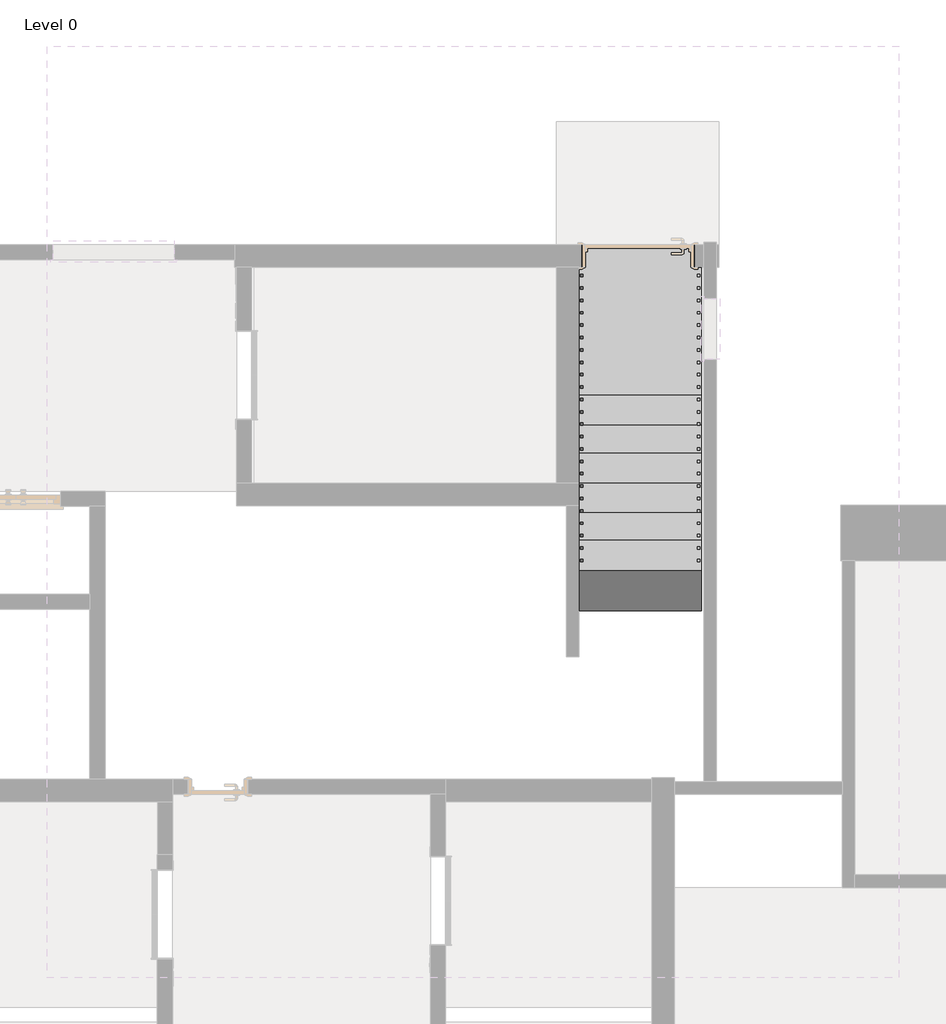
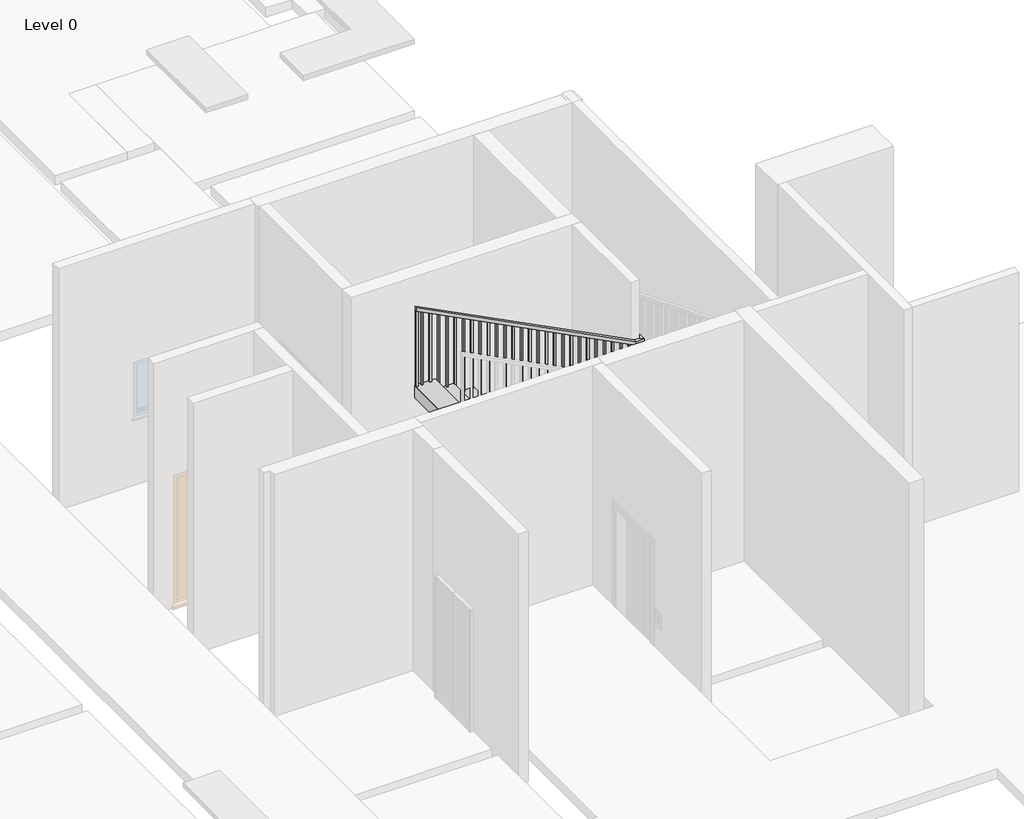
# One storey, part 12 of 14: 1 railing, 1 stair flight.
"""IFC4 building model written with IfcOpenShell, lengths in millimetres."""

from ifc_helpers import new_model, si_unit, frame, origin, place, context, project, spatial, polyline, outline, extrude, faceted_brep, element, save

model = new_model("IFC4")

# Units and contexts
model_context = context("Model", 3, world=origin())
ifc_project = project(units=[si_unit("LENGTHUNIT", "METRE", prefix="MILLI")], contexts=[model_context])

# Site, building, storey
site = spatial("IfcSite", under=ifc_project)
building = spatial("IfcBuilding", under=site)
storey = spatial("IfcBuildingStorey", under=building, Name="Level 0", Elevation=0.0)

# Railing
placement = place(None, origin())
element("IfcRailing", 1, ObjectType="1100mm", at=placement, inside=storey, context=model_context, shape_type="SolidModel", body=[
    faceted_brep([(-22529.0772109, 51059.2706597, 1266.6666667), (-22529.0772109, 51059.2706597, 1212.8024595), (-22579.0772109, 51059.2706597, 1212.8024595), (-22579.0772109, 51059.2706597, 1266.6666667), (-22529.0772109, 46974.2320599, 2903.4429161), (-22529.0772109, 46924.2320599, 2869.6125007), (-22579.0772109, 46924.2320599, 2869.6125007), (-22579.0772109, 46974.2320599, 2903.4429161), (-25957.6772109, 46849.2320599, 4766.6666667), (-25957.6772109, 46899.2320599, 4766.6666667), (-25957.6772109, 46899.2320599, 4710.4793192), (-25957.6772109, 46849.2320599, 4710.4793192), (-22666.1466162, 46849.2320599, 3023.0851989), (-22654.0772109, 46849.2320599, 3073.0851989), (-22666.1466162, 46899.2320599, 3023.0851989), (-22654.0772109, 46899.2320599, 3073.0851989), (-22529.0772109, 46974.2320599, 3073.0851989), (-22529.0772109, 46924.2320599, 3023.0851989), (-22579.0772109, 46924.2320599, 3023.0851989), (-22579.0772109, 46974.2320599, 3073.0851989), (-22529.0772109, 46849.2320599, 3073.0851989), (-22529.0772109, 46849.2320599, 3023.0851989), (-22579.0772109, 46899.2320599, 3023.0851989), (-22579.0772109, 46899.2320599, 3073.0851989)], [[[0, 1, 2, 3]], [[1, 0, 4, 5]], [[2, 1, 5, 6]], [[3, 2, 6, 7]], [[0, 3, 7, 4]], [[8, 9, 10, 11]], [[12, 13, 8, 11]], [[14, 12, 11, 10]], [[15, 14, 10, 9]], [[13, 15, 9, 8]], [[5, 4, 16, 17]], [[6, 5, 17, 18]], [[7, 6, 18, 19]], [[4, 7, 19, 16]], [[17, 16, 20, 21]], [[18, 17, 21, 22]], [[19, 18, 22, 23]], [[16, 19, 23, 20]], [[21, 20, 13, 12]], [[22, 21, 12, 14]], [[23, 22, 14, 15]], [[20, 23, 15, 13]]]),
    extrude(outline(polyline([(3500.0, -25854.0772109), (4657.3690637, -25854.0772109), (4670.185245, -25879.0772109), (3500.0, -25879.0772109), (3500.0, -25854.0772109)])), frame((0.0, 46861.7320599, 0.0), z_axis=(0.0, 1.0, 0.0), x_axis=(0.0, 0.0, 1.0)), (0.0, 0.0, 1.0), 25.0),
    extrude(outline(polyline([(3500.0, -25729.0772109), (4593.288157, -25729.0772109), (4606.1043383, -25754.0772109), (3500.0, -25754.0772109), (3500.0, -25729.0772109)])), frame((0.0, 46861.7320599, 0.0), z_axis=(0.0, 1.0, 0.0), x_axis=(0.0, 0.0, 1.0)), (0.0, 0.0, 1.0), 25.0),
    extrude(outline(polyline([(3333.3333333, -25604.0772109), (4529.2072502, -25604.0772109), (4542.0234316, -25629.0772109), (3333.3333333, -25629.0772109), (3333.3333333, -25604.0772109)])), frame((0.0, 46861.7320599, 0.0), z_axis=(0.0, 1.0, 0.0), x_axis=(0.0, 0.0, 1.0)), (0.0, 0.0, 1.0), 25.0),
    extrude(outline(polyline([(3333.3333333, -25479.0772109), (4465.1263435, -25479.0772109), (4477.9425249, -25504.0772109), (3333.3333333, -25504.0772109), (3333.3333333, -25479.0772109)])), frame((0.0, 46861.7320599, 0.0), z_axis=(0.0, 1.0, 0.0), x_axis=(0.0, 0.0, 1.0)), (0.0, 0.0, 1.0), 25.0),
    extrude(outline(polyline([(3166.6666667, -25354.0772109), (4401.0454368, -25354.0772109), (4413.8616181, -25379.0772109), (3166.6666667, -25379.0772109), (3166.6666667, -25354.0772109)])), frame((0.0, 46861.7320599, 0.0), z_axis=(0.0, 1.0, 0.0), x_axis=(0.0, 0.0, 1.0)), (0.0, 0.0, 1.0), 25.0),
    extrude(outline(polyline([(3166.6666667, -25229.0772109), (4336.96453, -25229.0772109), (4349.7807114, -25254.0772109), (3166.6666667, -25254.0772109), (3166.6666667, -25229.0772109)])), frame((0.0, 46861.7320599, 0.0), z_axis=(0.0, 1.0, 0.0), x_axis=(0.0, 0.0, 1.0)), (0.0, 0.0, 1.0), 25.0),
    extrude(outline(polyline([(3166.6666667, -25104.0772109), (4272.8836233, -25104.0772109), (4285.6998047, -25129.0772109), (3166.6666667, -25129.0772109), (3166.6666667, -25104.0772109)])), frame((0.0, 46861.7320599, 0.0), z_axis=(0.0, 1.0, 0.0), x_axis=(0.0, 0.0, 1.0)), (0.0, 0.0, 1.0), 25.0),
    extrude(outline(polyline([(3000.0, -24979.0772109), (4208.8027166, -24979.0772109), (4221.6188979, -25004.0772109), (3000.0, -25004.0772109), (3000.0, -24979.0772109)])), frame((0.0, 46861.7320599, 0.0), z_axis=(0.0, 1.0, 0.0), x_axis=(0.0, 0.0, 1.0)), (0.0, 0.0, 1.0), 25.0),
    extrude(outline(polyline([(3000.0, -24854.0772109), (4144.7218099, -24854.0772109), (4157.5379912, -24879.0772109), (3000.0, -24879.0772109), (3000.0, -24854.0772109)])), frame((0.0, 46861.7320599, 0.0), z_axis=(0.0, 1.0, 0.0), x_axis=(0.0, 0.0, 1.0)), (0.0, 0.0, 1.0), 25.0),
    extrude(outline(polyline([(2833.3333333, -24729.0772109), (4080.6409031, -24729.0772109), (4093.4570845, -24754.0772109), (2833.3333333, -24754.0772109), (2833.3333333, -24729.0772109)])), frame((0.0, 46861.7320599, 0.0), z_axis=(0.0, 1.0, 0.0), x_axis=(0.0, 0.0, 1.0)), (0.0, 0.0, 1.0), 25.0),
    extrude(outline(polyline([(2833.3333333, -24604.0772109), (4016.5599964, -24604.0772109), (4029.3761778, -24629.0772109), (2833.3333333, -24629.0772109), (2833.3333333, -24604.0772109)])), frame((0.0, 46861.7320599, 0.0), z_axis=(0.0, 1.0, 0.0), x_axis=(0.0, 0.0, 1.0)), (0.0, 0.0, 1.0), 25.0),
    extrude(outline(polyline([(2833.3333333, -24479.0772109), (3952.4790897, -24479.0772109), (3965.295271, -24504.0772109), (2833.3333333, -24504.0772109), (2833.3333333, -24479.0772109)])), frame((0.0, 46861.7320599, 0.0), z_axis=(0.0, 1.0, 0.0), x_axis=(0.0, 0.0, 1.0)), (0.0, 0.0, 1.0), 25.0),
    extrude(outline(polyline([(2666.6666667, -24354.0772109), (3888.398183, -24354.0772109), (3901.2143643, -24379.0772109), (2666.6666667, -24379.0772109), (2666.6666667, -24354.0772109)])), frame((0.0, 46861.7320599, 0.0), z_axis=(0.0, 1.0, 0.0), x_axis=(0.0, 0.0, 1.0)), (0.0, 0.0, 1.0), 25.0),
    extrude(outline(polyline([(2666.6666667, -24229.0772109), (3824.3172762, -24229.0772109), (3837.1334576, -24254.0772109), (2666.6666667, -24254.0772109), (2666.6666667, -24229.0772109)])), frame((0.0, 46861.7320599, 0.0), z_axis=(0.0, 1.0, 0.0), x_axis=(0.0, 0.0, 1.0)), (0.0, 0.0, 1.0), 25.0),
    extrude(outline(polyline([(2500.0, -24104.0772109), (3760.2363695, -24104.0772109), (3773.0525508, -24129.0772109), (2500.0, -24129.0772109), (2500.0, -24104.0772109)])), frame((0.0, 46861.7320599, 0.0), z_axis=(0.0, 1.0, 0.0), x_axis=(0.0, 0.0, 1.0)), (0.0, 0.0, 1.0), 25.0),
    extrude(outline(polyline([(2500.0, -23979.0772109), (3696.1554628, -23979.0772109), (3708.9716441, -24004.0772109), (2500.0, -24004.0772109), (2500.0, -23979.0772109)])), frame((0.0, 46861.7320599, 0.0), z_axis=(0.0, 1.0, 0.0), x_axis=(0.0, 0.0, 1.0)), (0.0, 0.0, 1.0), 25.0),
    extrude(outline(polyline([(2333.3333333, -23854.0772109), (3632.074556, -23854.0772109), (3644.8907374, -23879.0772109), (2333.3333333, -23879.0772109), (2333.3333333, -23854.0772109)])), frame((0.0, 46861.7320599, 0.0), z_axis=(0.0, 1.0, 0.0), x_axis=(0.0, 0.0, 1.0)), (0.0, 0.0, 1.0), 25.0),
    extrude(outline(polyline([(2333.3333333, -23729.0772109), (3567.9936493, -23729.0772109), (3580.8098307, -23754.0772109), (2333.3333333, -23754.0772109), (2333.3333333, -23729.0772109)])), frame((0.0, 46861.7320599, 0.0), z_axis=(0.0, 1.0, 0.0), x_axis=(0.0, 0.0, 1.0)), (0.0, 0.0, 1.0), 25.0),
    extrude(outline(polyline([(2333.3333333, -23604.0772109), (3503.9127426, -23604.0772109), (3516.7289239, -23629.0772109), (2333.3333333, -23629.0772109), (2333.3333333, -23604.0772109)])), frame((0.0, 46861.7320599, 0.0), z_axis=(0.0, 1.0, 0.0), x_axis=(0.0, 0.0, 1.0)), (0.0, 0.0, 1.0), 25.0),
    extrude(outline(polyline([(2166.6666667, -23479.0772109), (3439.8318359, -23479.0772109), (3452.6480172, -23504.0772109), (2166.6666667, -23504.0772109), (2166.6666667, -23479.0772109)])), frame((0.0, 46861.7320599, 0.0), z_axis=(0.0, 1.0, 0.0), x_axis=(0.0, 0.0, 1.0)), (0.0, 0.0, 1.0), 25.0),
    extrude(outline(polyline([(2166.6666667, -23354.0772109), (3375.7509291, -23354.0772109), (3388.5671105, -23379.0772109), (2166.6666667, -23379.0772109), (2166.6666667, -23354.0772109)])), frame((0.0, 46861.7320599, 0.0), z_axis=(0.0, 1.0, 0.0), x_axis=(0.0, 0.0, 1.0)), (0.0, 0.0, 1.0), 25.0),
    extrude(outline(polyline([(2166.6666667, -23229.0772109), (3311.6700224, -23229.0772109), (3324.4862037, -23254.0772109), (2166.6666667, -23254.0772109), (2166.6666667, -23229.0772109)])), frame((0.0, 46861.7320599, 0.0), z_axis=(0.0, 1.0, 0.0), x_axis=(0.0, 0.0, 1.0)), (0.0, 0.0, 1.0), 25.0),
    extrude(outline(polyline([(2166.6666667, -23104.0772109), (3247.5891157, -23104.0772109), (3260.405297, -23129.0772109), (2166.6666667, -23129.0772109), (2166.6666667, -23104.0772109)])), frame((0.0, 46861.7320599, 0.0), z_axis=(0.0, 1.0, 0.0), x_axis=(0.0, 0.0, 1.0)), (0.0, 0.0, 1.0), 25.0),
    extrude(outline(polyline([(2000.0, -22979.0772109), (3183.5082089, -22979.0772109), (3196.3243903, -23004.0772109), (2000.0, -23004.0772109), (2000.0, -22979.0772109)])), frame((0.0, 46861.7320599, 0.0), z_axis=(0.0, 1.0, 0.0), x_axis=(0.0, 0.0, 1.0)), (0.0, 0.0, 1.0), 25.0),
    extrude(outline(polyline([(2000.0, -22854.0772109), (3119.4273022, -22854.0772109), (3132.2434836, -22879.0772109), (2000.0, -22879.0772109), (2000.0, -22854.0772109)])), frame((0.0, 46861.7320599, 0.0), z_axis=(0.0, 1.0, 0.0), x_axis=(0.0, 0.0, 1.0)), (0.0, 0.0, 1.0), 25.0),
    extrude(outline(polyline([(2000.0, -22729.0772109), (3055.3463955, -22729.0772109), (3068.1625768, -22754.0772109), (2000.0, -22754.0772109), (2000.0, -22729.0772109)])), frame((0.0, 46861.7320599, 0.0), z_axis=(0.0, 1.0, 0.0), x_axis=(0.0, 0.0, 1.0)), (0.0, 0.0, 1.0), 25.0),
    extrude(outline(polyline([(-22604.0772109, 46886.7320599), (-22604.0772109, 46861.7320599), (-22629.0772109, 46861.7320599), (-22629.0772109, 46886.7320599), (-22604.0772109, 46886.7320599)])), frame((0.0, 0.0, 1833.3333333), z_axis=(0.0, 0.0, 1.0), x_axis=(1.0, 0.0, 0.0)), (0.0, 0.0, 1.0), 1189.7518656),
    extrude(outline(polyline([(47009.2706597, 2835.5395887), (47009.2706597, 1666.6666667), (46984.2706597, 1666.6666667), (46984.2706597, 2845.5564846), (47009.2706597, 2835.5395887)])), frame((-22566.5772109, 0.0, 0.0), z_axis=(1.0, 0.0, 0.0), x_axis=(0.0, 1.0, 0.0)), (0.0, 0.0, 1.0), 25.0),
    extrude(outline(polyline([(47134.2706597, 2785.4551094), (47134.2706597, 1666.6666667), (47109.2706597, 1666.6666667), (47109.2706597, 2795.4720053), (47134.2706597, 2785.4551094)])), frame((-22566.5772109, 0.0, 0.0), z_axis=(1.0, 0.0, 0.0), x_axis=(0.0, 1.0, 0.0)), (0.0, 0.0, 1.0), 25.0),
    extrude(outline(polyline([(47259.2706597, 2735.3706301), (47259.2706597, 1500.0), (47234.2706597, 1500.0), (47234.2706597, 2745.387526), (47259.2706597, 2735.3706301)])), frame((-22566.5772109, 0.0, 0.0), z_axis=(1.0, 0.0, 0.0), x_axis=(0.0, 1.0, 0.0)), (0.0, 0.0, 1.0), 25.0),
    extrude(outline(polyline([(47384.2706597, 2685.2861508), (47384.2706597, 1500.0), (47359.2706597, 1500.0), (47359.2706597, 2695.3030467), (47384.2706597, 2685.2861508)])), frame((-22566.5772109, 0.0, 0.0), z_axis=(1.0, 0.0, 0.0), x_axis=(0.0, 1.0, 0.0)), (0.0, 0.0, 1.0), 25.0),
    extrude(outline(polyline([(47509.2706597, 2635.2016715), (47509.2706597, 1333.3333333), (47484.2706597, 1333.3333333), (47484.2706597, 2645.2185674), (47509.2706597, 2635.2016715)])), frame((-22566.5772109, 0.0, 0.0), z_axis=(1.0, 0.0, 0.0), x_axis=(0.0, 1.0, 0.0)), (0.0, 0.0, 1.0), 25.0),
    extrude(outline(polyline([(47634.2706597, 2585.1171922), (47634.2706597, 1333.3333333), (47609.2706597, 1333.3333333), (47609.2706597, 2595.1340881), (47634.2706597, 2585.1171922)])), frame((-22566.5772109, 0.0, 0.0), z_axis=(1.0, 0.0, 0.0), x_axis=(0.0, 1.0, 0.0)), (0.0, 0.0, 1.0), 25.0),
    extrude(outline(polyline([(47759.2706597, 2535.0327129), (47759.2706597, 1333.3333333), (47734.2706597, 1333.3333333), (47734.2706597, 2545.0496088), (47759.2706597, 2535.0327129)])), frame((-22566.5772109, 0.0, 0.0), z_axis=(1.0, 0.0, 0.0), x_axis=(0.0, 1.0, 0.0)), (0.0, 0.0, 1.0), 25.0),
    extrude(outline(polyline([(47884.2706597, 2484.9482337), (47884.2706597, 1166.6666667), (47859.2706597, 1166.6666667), (47859.2706597, 2494.9651295), (47884.2706597, 2484.9482337)])), frame((-22566.5772109, 0.0, 0.0), z_axis=(1.0, 0.0, 0.0), x_axis=(0.0, 1.0, 0.0)), (0.0, 0.0, 1.0), 25.0),
    extrude(outline(polyline([(48009.2706597, 2434.8637544), (48009.2706597, 1166.6666667), (47984.2706597, 1166.6666667), (47984.2706597, 2444.8806502), (48009.2706597, 2434.8637544)])), frame((-22566.5772109, 0.0, 0.0), z_axis=(1.0, 0.0, 0.0), x_axis=(0.0, 1.0, 0.0)), (0.0, 0.0, 1.0), 25.0),
    extrude(outline(polyline([(48134.2706597, 2384.7792751), (48134.2706597, 1000.0), (48109.2706597, 1000.0), (48109.2706597, 2394.7961709), (48134.2706597, 2384.7792751)])), frame((-22566.5772109, 0.0, 0.0), z_axis=(1.0, 0.0, 0.0), x_axis=(0.0, 1.0, 0.0)), (0.0, 0.0, 1.0), 25.0),
    extrude(outline(polyline([(48259.2706597, 2334.6947958), (48259.2706597, 1000.0), (48234.2706597, 1000.0), (48234.2706597, 2344.7116916), (48259.2706597, 2334.6947958)])), frame((-22566.5772109, 0.0, 0.0), z_axis=(1.0, 0.0, 0.0), x_axis=(0.0, 1.0, 0.0)), (0.0, 0.0, 1.0), 25.0),
    extrude(outline(polyline([(48384.2706597, 2284.6103165), (48384.2706597, 833.3333333), (48359.2706597, 833.3333333), (48359.2706597, 2294.6272123), (48384.2706597, 2284.6103165)])), frame((-22566.5772109, 0.0, 0.0), z_axis=(1.0, 0.0, 0.0), x_axis=(0.0, 1.0, 0.0)), (0.0, 0.0, 1.0), 25.0),
    extrude(outline(polyline([(48509.2706597, 2234.5258372), (48509.2706597, 833.3333333), (48484.2706597, 833.3333333), (48484.2706597, 2244.542733), (48509.2706597, 2234.5258372)])), frame((-22566.5772109, 0.0, 0.0), z_axis=(1.0, 0.0, 0.0), x_axis=(0.0, 1.0, 0.0)), (0.0, 0.0, 1.0), 25.0),
    extrude(outline(polyline([(48634.2706597, 2184.4413579), (48634.2706597, 833.3333333), (48609.2706597, 833.3333333), (48609.2706597, 2194.4582537), (48634.2706597, 2184.4413579)])), frame((-22566.5772109, 0.0, 0.0), z_axis=(1.0, 0.0, 0.0), x_axis=(0.0, 1.0, 0.0)), (0.0, 0.0, 1.0), 25.0),
    extrude(outline(polyline([(48759.2706597, 2134.3568786), (48759.2706597, 666.6666667), (48734.2706597, 666.6666667), (48734.2706597, 2144.3737744), (48759.2706597, 2134.3568786)])), frame((-22566.5772109, 0.0, 0.0), z_axis=(1.0, 0.0, 0.0), x_axis=(0.0, 1.0, 0.0)), (0.0, 0.0, 1.0), 25.0),
    extrude(outline(polyline([(48884.2706597, 2084.2723993), (48884.2706597, 666.6666667), (48859.2706597, 666.6666667), (48859.2706597, 2094.2892951), (48884.2706597, 2084.2723993)])), frame((-22566.5772109, 0.0, 0.0), z_axis=(1.0, 0.0, 0.0), x_axis=(0.0, 1.0, 0.0)), (0.0, 0.0, 1.0), 25.0),
    extrude(outline(polyline([(49009.2706597, 2034.18792), (49009.2706597, 500.0), (48984.2706597, 500.0), (48984.2706597, 2044.2048158), (49009.2706597, 2034.18792)])), frame((-22566.5772109, 0.0, 0.0), z_axis=(1.0, 0.0, 0.0), x_axis=(0.0, 1.0, 0.0)), (0.0, 0.0, 1.0), 25.0),
    extrude(outline(polyline([(49134.2706597, 1984.1034407), (49134.2706597, 500.0), (49109.2706597, 500.0), (49109.2706597, 1994.1203365), (49134.2706597, 1984.1034407)])), frame((-22566.5772109, 0.0, 0.0), z_axis=(1.0, 0.0, 0.0), x_axis=(0.0, 1.0, 0.0)), (0.0, 0.0, 1.0), 25.0),
    extrude(outline(polyline([(49259.2706597, 1934.0189614), (49259.2706597, 333.3333333), (49234.2706597, 333.3333333), (49234.2706597, 1944.0358573), (49259.2706597, 1934.0189614)])), frame((-22566.5772109, 0.0, 0.0), z_axis=(1.0, 0.0, 0.0), x_axis=(0.0, 1.0, 0.0)), (0.0, 0.0, 1.0), 25.0),
    extrude(outline(polyline([(49384.2706597, 1883.9344821), (49384.2706597, 333.3333333), (49359.2706597, 333.3333333), (49359.2706597, 1893.951378), (49384.2706597, 1883.9344821)])), frame((-22566.5772109, 0.0, 0.0), z_axis=(1.0, 0.0, 0.0), x_axis=(0.0, 1.0, 0.0)), (0.0, 0.0, 1.0), 25.0),
    extrude(outline(polyline([(49509.2706597, 1833.8500028), (49509.2706597, 333.3333333), (49484.2706597, 333.3333333), (49484.2706597, 1843.8668987), (49509.2706597, 1833.8500028)])), frame((-22566.5772109, 0.0, 0.0), z_axis=(1.0, 0.0, 0.0), x_axis=(0.0, 1.0, 0.0)), (0.0, 0.0, 1.0), 25.0),
    extrude(outline(polyline([(49634.2706597, 1783.7655235), (49634.2706597, 166.6666667), (49609.2706597, 166.6666667), (49609.2706597, 1793.7824194), (49634.2706597, 1783.7655235)])), frame((-22566.5772109, 0.0, 0.0), z_axis=(1.0, 0.0, 0.0), x_axis=(0.0, 1.0, 0.0)), (0.0, 0.0, 1.0), 25.0),
    extrude(outline(polyline([(49759.2706597, 1733.6810442), (49759.2706597, 166.6666667), (49734.2706597, 166.6666667), (49734.2706597, 1743.6979401), (49759.2706597, 1733.6810442)])), frame((-22566.5772109, 0.0, 0.0), z_axis=(1.0, 0.0, 0.0), x_axis=(0.0, 1.0, 0.0)), (0.0, 0.0, 1.0), 25.0),
    extrude(outline(polyline([(49884.2706597, 1683.5965649), (49884.2706597, 166.6666667), (49859.2706597, 166.6666667), (49859.2706597, 1693.6134608), (49884.2706597, 1683.5965649)])), frame((-22566.5772109, 0.0, 0.0), z_axis=(1.0, 0.0, 0.0), x_axis=(0.0, 1.0, 0.0)), (0.0, 0.0, 1.0), 25.0),
    extrude(outline(polyline([(50009.2706597, 1633.5120856), (50009.2706597, 166.6666667), (49984.2706597, 166.6666667), (49984.2706597, 1643.5289815), (50009.2706597, 1633.5120856)])), frame((-22566.5772109, 0.0, 0.0), z_axis=(1.0, 0.0, 0.0), x_axis=(0.0, 1.0, 0.0)), (0.0, 0.0, 1.0), 25.0),
    extrude(outline(polyline([(50134.2706597, 1583.4276063), (50134.2706597, 166.6666667), (50109.2706597, 166.6666667), (50109.2706597, 1593.4445022), (50134.2706597, 1583.4276063)])), frame((-22566.5772109, 0.0, 0.0), z_axis=(1.0, 0.0, 0.0), x_axis=(0.0, 1.0, 0.0)), (0.0, 0.0, 1.0), 25.0),
    extrude(outline(polyline([(50259.2706597, 1533.343127), (50259.2706597, 166.6666667), (50234.2706597, 166.6666667), (50234.2706597, 1543.3600229), (50259.2706597, 1533.343127)])), frame((-22566.5772109, 0.0, 0.0), z_axis=(1.0, 0.0, 0.0), x_axis=(0.0, 1.0, 0.0)), (0.0, 0.0, 1.0), 25.0),
    extrude(outline(polyline([(50384.2706597, 1483.2586477), (50384.2706597, 166.6666667), (50359.2706597, 166.6666667), (50359.2706597, 1493.2755436), (50384.2706597, 1483.2586477)])), frame((-22566.5772109, 0.0, 0.0), z_axis=(1.0, 0.0, 0.0), x_axis=(0.0, 1.0, 0.0)), (0.0, 0.0, 1.0), 25.0),
    extrude(outline(polyline([(50509.2706597, 1433.1741684), (50509.2706597, 166.6666667), (50484.2706597, 166.6666667), (50484.2706597, 1443.1910643), (50509.2706597, 1433.1741684)])), frame((-22566.5772109, 0.0, 0.0), z_axis=(1.0, 0.0, 0.0), x_axis=(0.0, 1.0, 0.0)), (0.0, 0.0, 1.0), 25.0),
    extrude(outline(polyline([(50634.2706597, 1383.0896891), (50634.2706597, 166.6666667), (50609.2706597, 166.6666667), (50609.2706597, 1393.106585), (50634.2706597, 1383.0896891)])), frame((-22566.5772109, 0.0, 0.0), z_axis=(1.0, 0.0, 0.0), x_axis=(0.0, 1.0, 0.0)), (0.0, 0.0, 1.0), 25.0),
    extrude(outline(polyline([(50759.2706597, 1333.0052098), (50759.2706597, 166.6666667), (50734.2706597, 166.6666667), (50734.2706597, 1343.0221057), (50759.2706597, 1333.0052098)])), frame((-22566.5772109, 0.0, 0.0), z_axis=(1.0, 0.0, 0.0), x_axis=(0.0, 1.0, 0.0)), (0.0, 0.0, 1.0), 25.0),
    extrude(outline(polyline([(50884.2706597, 1282.9207305), (50884.2706597, 166.6666667), (50859.2706597, 166.6666667), (50859.2706597, 1292.9376264), (50884.2706597, 1282.9207305)])), frame((-22566.5772109, 0.0, 0.0), z_axis=(1.0, 0.0, 0.0), x_axis=(0.0, 1.0, 0.0)), (0.0, 0.0, 1.0), 25.0),
    extrude(outline(polyline([(51009.2706597, 1232.8362512), (51009.2706597, 166.6666667), (50984.2706597, 166.6666667), (50984.2706597, 1242.8531471), (51009.2706597, 1232.8362512)])), frame((-22566.5772109, 0.0, 0.0), z_axis=(1.0, 0.0, 0.0), x_axis=(0.0, 1.0, 0.0)), (0.0, 0.0, 1.0), 25.0),
    extrude(outline(polyline([(-22566.5772109, 46886.7320599), (-22541.5772109, 46886.7320599), (-22541.5772109, 46861.7320599), (-22566.5772109, 46861.7320599), (-22566.5772109, 46886.7320599)])), frame((0.0, 0.0, 1833.3333333), z_axis=(0.0, 0.0, 1.0), x_axis=(1.0, 0.0, 0.0)), (0.0, 0.0, 1.0), 1189.7518656),
    extrude(outline(polyline([(3500.0, -25932.6772109), (4697.6631378, -25932.6772109), (4710.4793192, -25957.6772109), (3500.0, -25957.6772109), (3500.0, -25932.6772109)])), frame((0.0, 46861.7320599, 0.0), z_axis=(0.0, 1.0, 0.0), x_axis=(0.0, 0.0, 1.0)), (0.0, 0.0, 1.0), 25.0),
    extrude(outline(polyline([(51059.2706597, 1212.8024595), (51059.2706597, 166.6666667), (51034.2706597, 166.6666667), (51034.2706597, 1222.8193554), (51059.2706597, 1212.8024595)])), frame((-22566.5772109, 0.0, 0.0), z_axis=(1.0, 0.0, 0.0), x_axis=(0.0, 1.0, 0.0)), (0.0, 0.0, 1.0), 25.0),
])

# Stair flight
element("IfcStairFlight", 2, ObjectType="1mm_Tread-175mm_Depth", at=placement, inside=storey, context=model_context, shape_type="SolidModel", body=[
    faceted_brep([(-21345.2288686, 49541.2320599, 165.6666667), (-21345.2288686, 51059.2706597, 165.6666667), (-22579.4772109, 51059.2706597, 165.6666667), (-22579.4772109, 49541.2320599, 165.6666667), (-21345.2288686, 49541.2320599, 0.0), (-21345.2288686, 51059.2706597, 0.0), (-22579.4772109, 51059.2706597, 0.0), (-22579.4772109, 49541.2320599, 0.0), (-21345.2288686, 49541.2320599, 332.3333333), (-22579.4772109, 49541.2320599, 332.3333333), (-22579.4772109, 49495.01215, 332.3333333), (-22579.4772109, 49236.4320599, 332.3333333), (-21345.2288686, 49236.4320599, 332.3333333), (-21345.2288686, 49495.01215, 332.3333333), (-21345.2288686, 49236.4320599, 137.4981836), (-21345.2288686, 49478.5755278, 0.0), (-21345.2288686, 49495.01215, 0.0), (-22579.4772109, 49495.01215, 0.0), (-22579.4772109, 49478.5755278, 0.0), (-22579.4772109, 49236.4320599, 137.4981836), (-21345.2288686, 48954.0513598, 499.0), (-21345.2288686, 49236.4320599, 499.0), (-22579.4772109, 49236.4320599, 499.0), (-22579.4772109, 48954.0513598, 499.0), (-21345.2288686, 48954.0513598, 297.8445836), (-22579.4772109, 48954.0513598, 297.8445836), (-21345.2288686, 48352.6143129, 832.3333333), (-21345.2288686, 48652.2320599, 832.3333333), (-22579.4772109, 48652.2320599, 832.3333333), (-22579.4772109, 48352.6143129, 832.3333333), (-21345.2288686, 48352.6143129, 639.3631974), (-21345.2288686, 48652.2320599, 469.2289528), (-21345.2288686, 48652.2320599, 665.6666667), (-22579.4772109, 48652.2320599, 665.6666667), (-22579.4772109, 48652.2320599, 469.2289528), (-22579.4772109, 48352.6143129, 639.3631974), (-21345.2288686, 48073.3159129, 999.0), (-21345.2288686, 48352.6143129, 999.0), (-22579.4772109, 48352.6143129, 999.0), (-22579.4772109, 48073.3159129, 999.0), (-21345.2288686, 48073.3159129, 797.9593512), (-22579.4772109, 48073.3159129, 797.9593512), (-21345.2288686, 47184.3159129, 1499.0), (-21345.2288686, 47463.7159129, 1499.0), (-22579.4772109, 47463.7159129, 1499.0), (-22579.4772109, 47184.3159129, 1499.0), (-21345.2288686, 47184.3159129, 1302.7670435), (-21345.2288686, 47463.7159129, 1144.1131974), (-21345.2288686, 47463.7159129, 1332.3333333), (-22579.4772109, 47463.7159129, 1332.3333333), (-22579.4772109, 47463.7159129, 1144.1131974), (-22579.4772109, 47184.3159129, 1302.7670435), (-21345.2288686, 46899.6320599, 1665.6666667), (-21345.2288686, 47184.3159129, 1665.6666667), (-22579.4772109, 47184.3159129, 1665.6666667), (-22579.4772109, 46899.6320599, 1665.6666667), (-21345.2288686, 46899.6320599, 1464.4212605), (-22579.4772109, 46559.9010389, 1657.3333333), (-22579.4772109, 46899.6320599, 1657.3333333), (-22706.5788109, 45661.6690597, 1832.3333333), (-21345.2288686, 45661.6690597, 1832.3333333), (-21345.2288686, 46559.9010389, 1832.3333333), (-21345.2288686, 46899.6320599, 1832.3333333), (-22579.4772109, 46899.6320599, 1832.3333333), (-22706.5788109, 46899.6320599, 1832.3333333), (-22706.5788109, 45661.6690597, 1824.0), (-22706.5788109, 45661.6690597, 1657.3333333), (-21345.2288686, 45661.6690597, 1657.3333333), (-22706.5788109, 46899.6320599, 1657.3333333), (-22706.5788109, 46899.6320599, 1824.0), (-23011.3788109, 45661.6690597, 1999.0), (-22706.5788109, 45661.6690597, 1999.0), (-22706.5788109, 46899.6320599, 1999.0), (-23011.3788109, 46899.6320599, 1999.0), (-23011.3788109, 45661.6690597, 1990.6666667), (-23011.3788109, 45661.6690597, 1824.0), (-23011.3788109, 46899.6320599, 1824.0), (-23011.3788109, 46899.6320599, 1990.6666667), (-23597.5805211, 45661.6690597, 2165.6666667), (-23011.3788109, 45661.6690597, 2165.6666667), (-23011.3788109, 46899.6320599, 2165.6666667), (-23597.5805211, 46899.6320599, 2165.6666667), (-23597.5805211, 45661.6690597, 1990.6666667), (-23597.5805211, 46899.6320599, 1990.6666667), (-23597.5805211, 45661.6690597, 2332.3333333), (-23597.5805211, 46899.6320599, 2332.3333333), (-23643.7452835, 46899.6320599, 2332.3333333), (-23876.9805211, 46899.6320599, 2332.3333333), (-23876.9805211, 45661.6690597, 2332.3333333), (-23643.7452835, 45661.6690597, 2332.3333333), (-23876.9805211, 45661.6690597, 2122.9247483), (-23643.7452835, 45661.6690597, 1990.6666667), (-23643.7452835, 46899.6320599, 1990.6666667), (-23876.9805211, 46899.6320599, 2122.9247483), (-24765.9805211, 45661.6690597, 2832.3333333), (-24486.5805211, 45661.6690597, 2832.3333333), (-24486.5805211, 46899.6320599, 2832.3333333), (-24765.9805211, 46899.6320599, 2832.3333333), (-24765.9805211, 45661.6690597, 2627.0399746), (-24486.5805211, 45661.6690597, 2468.6037606), (-24486.5805211, 45661.6690597, 2665.6666667), (-24486.5805211, 46899.6320599, 2665.6666667), (-24486.5805211, 46899.6320599, 2468.6037606), (-24765.9805211, 46899.6320599, 2627.0399746), (-25070.7805211, 45661.6690597, 2999.0), (-24765.9805211, 45661.6690597, 2999.0), (-24765.9805211, 46899.6320599, 2999.0), (-25070.7805211, 46899.6320599, 2999.0), (-25070.7805211, 45661.6690597, 2799.8794808), (-25070.7805211, 46899.6320599, 2799.8794808), (-25654.9805211, 45661.6690597, 3332.3333333), (-25375.5805211, 45661.6690597, 3332.3333333), (-25375.5805211, 46899.6320599, 3332.3333333), (-25654.9805211, 46899.6320599, 3332.3333333), (-25654.9805211, 45661.6690597, 3131.1552009), (-25375.5805211, 45661.6690597, 2972.718987), (-25375.5805211, 45661.6690597, 3165.6666667), (-25375.5805211, 46899.6320599, 3165.6666667), (-25375.5805211, 46899.6320599, 2972.718987), (-25654.9805211, 46899.6320599, 3131.1552009), (-25957.6772109, 45661.6690597, 3499.0), (-25654.9805211, 45661.6690597, 3499.0), (-25654.9805211, 46899.6320599, 3499.0), (-25957.6772109, 46899.6320599, 3499.0), (-25957.6772109, 45661.6690597, 3302.8020067), (-25957.6772109, 46899.6320599, 3302.8020067), (-21345.2288686, 46559.9010389, 1657.3333333), (-22579.4772109, 47768.5159129, 971.0362743), (-21345.2288686, 47768.5159129, 971.0362743), (-24181.7805211, 45661.6690597, 2295.7642544), (-24181.7805211, 46899.6320599, 2295.7642544), (-21345.2288686, 48954.0513598, 665.6666667), (-22579.4772109, 48954.0513598, 665.6666667), (-21345.2288686, 47768.5159129, 1165.6666667), (-21345.2288686, 48073.3159129, 1165.6666667), (-22579.4772109, 48073.3159129, 1165.6666667), (-22579.4772109, 47768.5159129, 1165.6666667), (-21345.2288686, 47768.5159129, 1332.3333333), (-22579.4772109, 47768.5159129, 1332.3333333), (-24181.7805211, 45661.6690597, 2499.0), (-23876.9805211, 45661.6690597, 2499.0), (-23876.9805211, 46899.6320599, 2499.0), (-24181.7805211, 46899.6320599, 2499.0), (-24181.7805211, 45661.6690597, 2665.6666667), (-24181.7805211, 46899.6320599, 2665.6666667), (-25070.7805211, 45661.6690597, 3165.6666667), (-25070.7805211, 46899.6320599, 3165.6666667)], [[[0, 1, 2, 3]], [[1, 0, 4, 5]], [[2, 1, 5, 6]], [[3, 2, 6, 7]], [[8, 9, 10, 11, 12, 13]], [[4, 0, 8, 13, 12, 14, 15, 16]], [[0, 3, 9, 8]], [[3, 7, 17, 18, 19, 11, 10, 9]], [[20, 21, 22, 23]], [[21, 20, 24, 14, 12]], [[12, 11, 22, 21]], [[23, 22, 11, 19, 25]], [[26, 27, 28, 29]], [[27, 26, 30, 31, 32]], [[32, 33, 28, 27]], [[29, 28, 33, 34, 35]], [[36, 37, 38, 39]], [[37, 36, 40, 30, 26]], [[26, 29, 38, 37]], [[39, 38, 29, 35, 41]], [[42, 43, 44, 45]], [[43, 42, 46, 47, 48]], [[48, 49, 44, 43]], [[45, 44, 49, 50, 51]], [[52, 53, 54, 55]], [[53, 52, 56, 46, 42]], [[42, 45, 54, 53]], [[55, 54, 45, 51, 57, 58]], [[59, 60, 61, 62, 63, 64]], [[60, 59, 65, 66, 67]], [[52, 55, 63, 62]], [[64, 63, 55, 58, 68, 69]], [[70, 71, 72, 73]], [[71, 70, 74, 75, 65, 59]], [[59, 64, 72, 71]], [[73, 72, 64, 69, 76, 77]], [[78, 79, 80, 81]], [[79, 78, 82, 74, 70]], [[70, 73, 80, 79]], [[81, 80, 73, 77, 83]], [[84, 85, 86, 87, 88, 89]], [[78, 84, 89, 88, 90, 91, 82]], [[78, 81, 85, 84]], [[85, 81, 83, 92, 93, 87, 86]], [[94, 95, 96, 97]], [[95, 94, 98, 99, 100]], [[100, 101, 96, 95]], [[97, 96, 101, 102, 103]], [[104, 105, 106, 107]], [[105, 104, 108, 98, 94]], [[94, 97, 106, 105]], [[107, 106, 97, 103, 109]], [[110, 111, 112, 113]], [[111, 110, 114, 115, 116]], [[116, 117, 112, 111]], [[113, 112, 117, 118, 119]], [[120, 121, 122, 123]], [[121, 120, 124, 114, 110]], [[110, 113, 122, 121]], [[123, 122, 113, 119, 125]], [[120, 123, 125, 124]], [[5, 4, 16, 15, 18, 17, 7, 6]], [[126, 57, 51, 50, 127, 41, 35, 34, 25, 19, 18, 15, 14, 24, 31, 30, 40, 128, 47, 46, 56]], [[66, 68, 58, 57, 126, 67]], [[75, 76, 69, 65]], [[77, 74, 82, 91, 92, 83]], [[92, 91, 90, 129, 99, 98, 108, 115, 114, 124, 125, 119, 118, 109, 103, 102, 130, 93]], [[32, 131, 132, 33]], [[131, 32, 31, 24, 20]], [[20, 23, 132, 131]], [[33, 132, 23, 25, 34]], [[133, 134, 135, 136]], [[134, 133, 128, 40, 36]], [[36, 39, 135, 134]], [[136, 135, 39, 41, 127]], [[48, 137, 138, 49]], [[137, 48, 47, 128, 133]], [[133, 136, 138, 137]], [[49, 138, 136, 127, 50]], [[52, 62, 61, 60, 67, 126, 56]], [[139, 140, 141, 142]], [[140, 139, 129, 90, 88]], [[88, 87, 141, 140]], [[142, 141, 87, 93, 130]], [[100, 143, 144, 101]], [[143, 100, 99, 129, 139]], [[139, 142, 144, 143]], [[101, 144, 142, 130, 102]], [[116, 145, 146, 117]], [[145, 116, 115, 108, 104]], [[104, 107, 146, 145]], [[117, 146, 107, 109, 118]], [[68, 66, 65, 69]], [[76, 75, 74, 77]]]),
    extrude(outline(polyline([(-21345.2288686, 49541.2320599), (-22579.4772109, 49541.2320599), (-22579.4772109, 51059.2706597), (-21345.2288686, 51059.2706597), (-21345.2288686, 49541.2320599)])), frame((0.0, 0.0, 165.6666667), z_axis=(0.0, 0.0, 1.0), x_axis=(1.0, 0.0, 0.0)), (0.0, 0.0, 1.0), 1.0),
    extrude(outline(polyline([(-21345.2288686, 49236.4320599), (-22579.4772109, 49236.4320599), (-22579.4772109, 49541.2320599), (-21345.2288686, 49541.2320599), (-21345.2288686, 49236.4320599)])), frame((0.0, 0.0, 332.3333333), z_axis=(0.0, 0.0, 1.0), x_axis=(1.0, 0.0, 0.0)), (0.0, 0.0, 1.0), 1.0),
    extrude(outline(polyline([(-21345.2288686, 48954.0513598), (-22579.4772109, 48954.0513598), (-22579.4772109, 49236.4320599), (-21345.2288686, 49236.4320599), (-21345.2288686, 48954.0513598)])), frame((0.0, 0.0, 499.0), z_axis=(0.0, 0.0, 1.0), x_axis=(1.0, 0.0, 0.0)), (0.0, 0.0, 1.0), 1.0),
    extrude(outline(polyline([(-21345.2288686, 48352.6143129), (-22579.4772109, 48352.6143129), (-22579.4772109, 48652.2320599), (-21345.2288686, 48652.2320599), (-21345.2288686, 48352.6143129)])), frame((0.0, 0.0, 832.3333333), z_axis=(0.0, 0.0, 1.0), x_axis=(1.0, 0.0, 0.0)), (0.0, 0.0, 1.0), 1.0),
    extrude(outline(polyline([(-21345.2288686, 48073.3159129), (-22579.4772109, 48073.3159129), (-22579.4772109, 48352.6143129), (-21345.2288686, 48352.6143129), (-21345.2288686, 48073.3159129)])), frame((0.0, 0.0, 999.0), z_axis=(0.0, 0.0, 1.0), x_axis=(1.0, 0.0, 0.0)), (0.0, 0.0, 1.0), 1.0),
    extrude(outline(polyline([(-21345.2288686, 47184.3159129), (-22579.4772109, 47184.3159129), (-22579.4772109, 47463.7159129), (-21345.2288686, 47463.7159129), (-21345.2288686, 47184.3159129)])), frame((0.0, 0.0, 1499.0), z_axis=(0.0, 0.0, 1.0), x_axis=(1.0, 0.0, 0.0)), (0.0, 0.0, 1.0), 1.0),
    extrude(outline(polyline([(-21345.2288686, 46899.6320599), (-22579.4772109, 46899.6320599), (-22579.4772109, 47184.3159129), (-21345.2288686, 47184.3159129), (-21345.2288686, 46899.6320599)])), frame((0.0, 0.0, 1665.6666667), z_axis=(0.0, 0.0, 1.0), x_axis=(1.0, 0.0, 0.0)), (0.0, 0.0, 1.0), 1.0),
    extrude(outline(polyline([(-22706.5788109, 45661.6690597), (-22706.5788109, 46899.6320599), (-22579.4772109, 46899.6320599), (-21345.2288686, 46899.6320599), (-21345.2288686, 45661.6690597), (-22706.5788109, 45661.6690597)])), frame((0.0, 0.0, 1832.3333333), z_axis=(0.0, 0.0, 1.0), x_axis=(1.0, 0.0, 0.0)), (0.0, 0.0, 1.0), 1.0),
    extrude(outline(polyline([(-23011.3788109, 45661.6690597), (-23011.3788109, 46899.6320599), (-22706.5788109, 46899.6320599), (-22706.5788109, 45661.6690597), (-23011.3788109, 45661.6690597)])), frame((0.0, 0.0, 1999.0), z_axis=(0.0, 0.0, 1.0), x_axis=(1.0, 0.0, 0.0)), (0.0, 0.0, 1.0), 1.0),
    extrude(outline(polyline([(-23597.5805211, 45661.6690597), (-23597.5805211, 46899.6320599), (-23011.3788109, 46899.6320599), (-23011.3788109, 45661.6690597), (-23597.5805211, 45661.6690597)])), frame((0.0, 0.0, 2165.6666667), z_axis=(0.0, 0.0, 1.0), x_axis=(1.0, 0.0, 0.0)), (0.0, 0.0, 1.0), 1.0),
    extrude(outline(polyline([(-23876.9805211, 45661.6690597), (-23876.9805211, 46899.6320599), (-23597.5805211, 46899.6320599), (-23597.5805211, 45661.6690597), (-23876.9805211, 45661.6690597)])), frame((0.0, 0.0, 2332.3333333), z_axis=(0.0, 0.0, 1.0), x_axis=(1.0, 0.0, 0.0)), (0.0, 0.0, 1.0), 1.0),
    extrude(outline(polyline([(-24765.9805211, 45661.6690597), (-24765.9805211, 46899.6320599), (-24486.5805211, 46899.6320599), (-24486.5805211, 45661.6690597), (-24765.9805211, 45661.6690597)])), frame((0.0, 0.0, 2832.3333333), z_axis=(0.0, 0.0, 1.0), x_axis=(1.0, 0.0, 0.0)), (0.0, 0.0, 1.0), 1.0),
    extrude(outline(polyline([(-25070.7805211, 45661.6690597), (-25070.7805211, 46899.6320599), (-24765.9805211, 46899.6320599), (-24765.9805211, 45661.6690597), (-25070.7805211, 45661.6690597)])), frame((0.0, 0.0, 2999.0), z_axis=(0.0, 0.0, 1.0), x_axis=(1.0, 0.0, 0.0)), (0.0, 0.0, 1.0), 1.0),
    extrude(outline(polyline([(-25654.9805211, 45661.6690597), (-25654.9805211, 46899.6320599), (-25375.5805211, 46899.6320599), (-25375.5805211, 45661.6690597), (-25654.9805211, 45661.6690597)])), frame((0.0, 0.0, 3332.3333333), z_axis=(0.0, 0.0, 1.0), x_axis=(1.0, 0.0, 0.0)), (0.0, 0.0, 1.0), 1.0),
    extrude(outline(polyline([(-25957.6772109, 45661.6690597), (-25957.6772109, 46899.6320599), (-25654.9805211, 46899.6320599), (-25654.9805211, 45661.6690597), (-25957.6772109, 45661.6690597)])), frame((0.0, 0.0, 3499.0), z_axis=(0.0, 0.0, 1.0), x_axis=(1.0, 0.0, 0.0)), (0.0, 0.0, 1.0), 1.0),
    extrude(outline(polyline([(-21345.2288686, 48652.2320599), (-22579.4772109, 48652.2320599), (-22579.4772109, 48954.0513598), (-21345.2288686, 48954.0513598), (-21345.2288686, 48652.2320599)])), frame((0.0, 0.0, 665.6666667), z_axis=(0.0, 0.0, 1.0), x_axis=(1.0, 0.0, 0.0)), (0.0, 0.0, 1.0), 1.0),
    extrude(outline(polyline([(-21345.2288686, 47768.5159129), (-22579.4772109, 47768.5159129), (-22579.4772109, 48073.3159129), (-21345.2288686, 48073.3159129), (-21345.2288686, 47768.5159129)])), frame((0.0, 0.0, 1165.6666667), z_axis=(0.0, 0.0, 1.0), x_axis=(1.0, 0.0, 0.0)), (0.0, 0.0, 1.0), 1.0),
    extrude(outline(polyline([(-21345.2288686, 47463.7159129), (-22579.4772109, 47463.7159129), (-22579.4772109, 47768.5159129), (-21345.2288686, 47768.5159129), (-21345.2288686, 47463.7159129)])), frame((0.0, 0.0, 1332.3333333), z_axis=(0.0, 0.0, 1.0), x_axis=(1.0, 0.0, 0.0)), (0.0, 0.0, 1.0), 1.0),
    extrude(outline(polyline([(-24181.7805211, 45661.6690597), (-24181.7805211, 46899.6320599), (-23876.9805211, 46899.6320599), (-23876.9805211, 45661.6690597), (-24181.7805211, 45661.6690597)])), frame((0.0, 0.0, 2499.0), z_axis=(0.0, 0.0, 1.0), x_axis=(1.0, 0.0, 0.0)), (0.0, 0.0, 1.0), 1.0),
    extrude(outline(polyline([(-24486.5805211, 45661.6690597), (-24486.5805211, 46899.6320599), (-24181.7805211, 46899.6320599), (-24181.7805211, 45661.6690597), (-24486.5805211, 45661.6690597)])), frame((0.0, 0.0, 2665.6666667), z_axis=(0.0, 0.0, 1.0), x_axis=(1.0, 0.0, 0.0)), (0.0, 0.0, 1.0), 1.0),
    extrude(outline(polyline([(-25375.5805211, 45661.6690597), (-25375.5805211, 46899.6320599), (-25070.7805211, 46899.6320599), (-25070.7805211, 45661.6690597), (-25375.5805211, 45661.6690597)])), frame((0.0, 0.0, 3165.6666667), z_axis=(0.0, 0.0, 1.0), x_axis=(1.0, 0.0, 0.0)), (0.0, 0.0, 1.0), 1.0),
])

save(model, "model.ifc")

# Revit data of these elements
# Type "1100mm"
#   built-in parameter 1008612 = 0.019685 (stored number, unit not read)
#   built-in parameter 1008611 = 0.019685 (stored number, unit not read)
#   built-in parameter 1008609 = 0.902231 (stored number, unit not read)
#   built-in parameter 1008604 = 0.19685 (stored number, unit not read)
#   built-in parameter 1008603 = 0.164042 (stored number, unit not read)
#   Railing Height = 1100 mm
#   built-in parameter 1008630 = 2
#   built-in parameter 1008610 = 2
#   built-in parameter 1008608 = 1
#   built-in parameter 1008618 = Baluster_Square : 25mm
# Element 1 (IfcRailing, "1100mm")
#   Phase Created = New Construction
# Element 2 (IfcStairFlight, "1mm_Tread-175mm_Depth")
#   Phase Created = New Construction
#   Materials on its faces: "Concrete, Cast-in-Place gray"
# Materials
#   "Concrete, Cast-in-Place gray": class "Concrete", colour RGB 192 192 192, transparency 0, Description = "Cast-in-place concrete", Cost = 0
